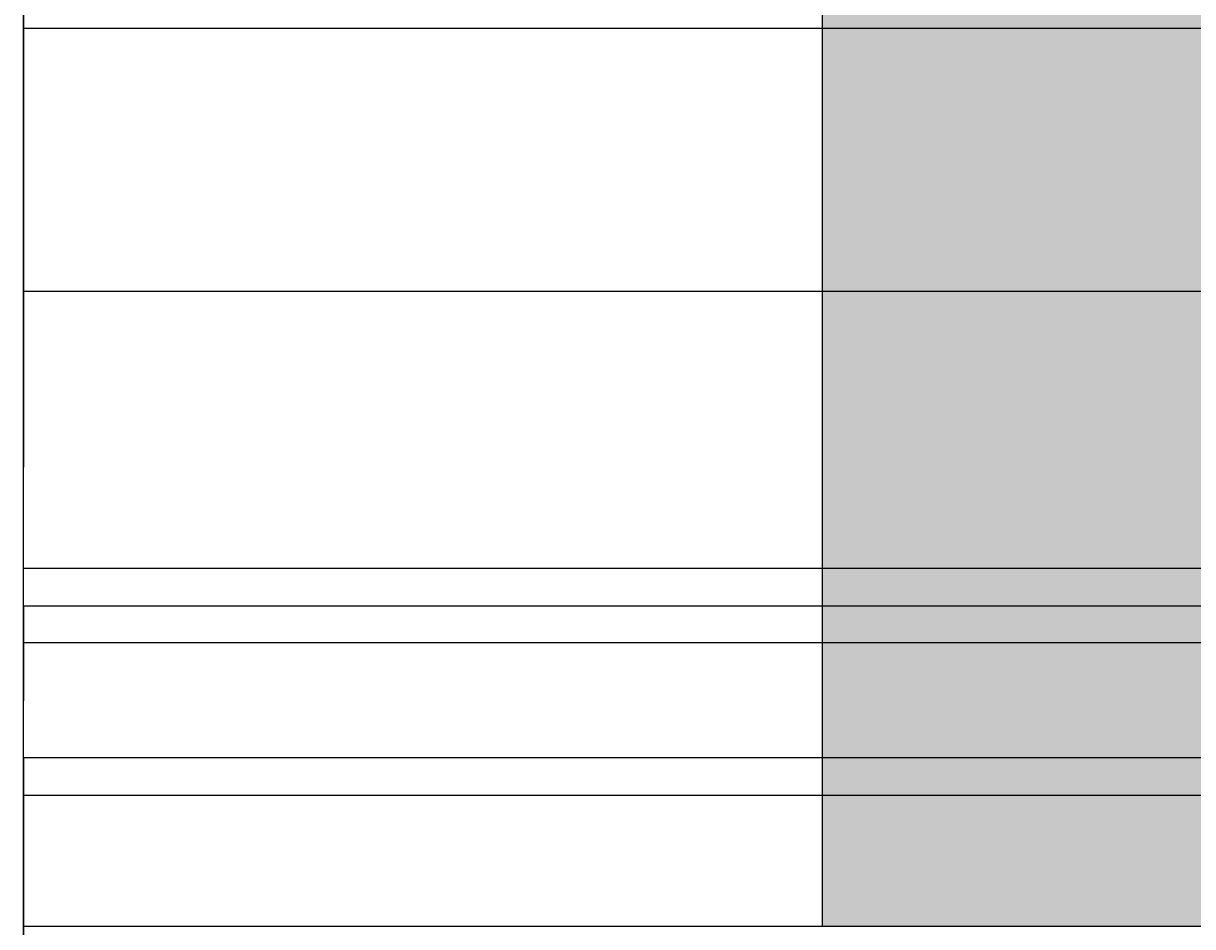
# Model space of a CAD drawing. Units: inches. Extents: x 35362 to 73946, y 43607 to 67532.
# Tile 3 of 134: x 35362 to 37937, y 46919 to 48909. Entities that reach past the tile are written whole.
import ezdxf

# ---------------------------------------------------------------- set-up
doc = ezdxf.new("R2010")
doc.units = ezdxf.units.IN
doc.header["$MEASUREMENT"] = 0
for name, color, linetype, lineweight in [('A-ANNO-DIMS', 2, 'Continuous', 18), ('E-SYMB', 1, 'Continuous', 25), ('E-SYMB-PATT', 1, 'Continuous', 13)]:
    doc.layers.add(name, color=color, linetype=linetype, lineweight=lineweight)
doc.styles.get("Standard").update_dxf_attribs({"font": 'arial.ttf'})
doc.dimstyles.get("Standard").update_dxf_attribs({"dimtxt": 0.18, "dimasz": 0.18, "dimexe": 0.18, "dimexo": 0.0625, "dimgap": 0.09, "dimtad": 0, "dimtih": 1, "dimtoh": 1, "dimdec": 4, "dimzin": 0, "dimdsep": 46, "dimtxsty": 'Standard', "dimcen": 0.09, "dimadec": 0, "dimazin": 0, "dimtfac": 1, "dimtdec": 4, "dimtofl": 0, "dimtmove": 0, "dimatfit": 3, "dimfxl": 1, "dimtolj": 1, "dimtzin": 0, "dimarcsym": 0})

# ---------------------------------------------------------------- blocks, each defined once
blk = doc.blocks.new('*D16')
at = {"layer": 'A-ANNO-DIMS', "color": 0, "lineweight": -2, "transparency": 16777216}
for p, q in [((37121.9, 49689.8), (35361.8, 49689.8)), ((35361.9, 49689.7), (35361.9, 48304.8)), ((35361.9, 46919.6), (35361.9, 48304.4)), ((37121.9, 46919.4), (35361.8, 46919.4))]:
    blk.add_line(p, q, dxfattribs=at)
at = {"layer": 'A-ANNO-DIMS', "color": 0, "transparency": 16777216}
for points in [[(35361.9, 49689.7), (35362, 49689.7), (35361.9, 49689.8)], [(35361.9, 46919.6), (35362, 46919.6), (35361.9, 46919.4)]]:
    blk.add_solid(points, dxfattribs=at)
at = {"layer": 'Defpoints', "color": 0, "transparency": 16777216}
for p in [(37121.9, 49689.8), (35361.9, 46919.4), (37121.9, 46919.4)]:
    blk.add_point(p, dxfattribs=at)
at = {"layer": 'A-ANNO-DIMS', "color": 0, "transparency": 16777216, "insert": (35361.9, 48304.6), "char_height": 0.18, "attachment_point": 5}
blk.add_mtext('\\A1;2770.5', dxfattribs=at)
blk = doc.blocks.new('*D43')
at = {"layer": 'A-ANNO-DIMS', "color": 0, "lineweight": -2, "transparency": 16777216}
for p, q in [((62004.7, 47625.2), (35361.8, 47625.2)), ((35361.9, 47625), (35361.9, 47416.9)), ((35361.9, 47208.4), (35361.9, 47416.5)), ((62004.7, 47208.2), (35361.8, 47208.2))]:
    blk.add_line(p, q, dxfattribs=at)
at = {"layer": 'A-ANNO-DIMS', "color": 0, "transparency": 16777216}
for points in [[(35361.9, 47625), (35362, 47625), (35361.9, 47625.2)], [(35361.9, 47208.4), (35362, 47208.4), (35361.9, 47208.2)]]:
    blk.add_solid(points, dxfattribs=at)
at = {"layer": 'Defpoints', "color": 0, "transparency": 16777216}
for p in [(62004.7, 47625.2), (35361.9, 47208.2), (62004.7, 47208.2)]:
    blk.add_point(p, dxfattribs=at)
at = {"layer": 'A-ANNO-DIMS', "color": 0, "transparency": 16777216, "insert": (35361.9, 47416.7), "char_height": 0.18, "attachment_point": 5}
blk.add_mtext('\\A1;416.9', dxfattribs=at)
blk = doc.blocks.new('*D67')
at = {"layer": 'A-ANNO-DIMS', "color": 0, "lineweight": -2, "transparency": 16777216}
for p, q in [((56873.5, 53351.5), (35361.8, 53351.5)), ((35361.9, 53351.3), (35361.9, 49400.9)), ((35361.9, 45450.1), (35361.9, 49400.5)), ((53793.6, 45449.9), (35361.8, 45449.9))]:
    blk.add_line(p, q, dxfattribs=at)
at = {"layer": 'A-ANNO-DIMS', "color": 0, "transparency": 16777216}
for points in [[(35361.9, 53351.3), (35362, 53351.3), (35361.9, 53351.5)], [(35361.9, 45450.1), (35362, 45450.1), (35361.9, 45449.9)]]:
    blk.add_solid(points, dxfattribs=at)
at = {"layer": 'Defpoints', "color": 0, "transparency": 16777216}
for p in [(35361.9, 53351.5), (56873.6, 53351.5), (53793.6, 45449.9)]:
    blk.add_point(p, dxfattribs=at)
at = {"layer": 'A-ANNO-DIMS', "color": 0, "transparency": 16777216, "insert": (35361.9, 49400.7), "char_height": 0.18, "attachment_point": 5}
blk.add_mtext('\\A1;7901.6', dxfattribs=at)
blk = doc.blocks.new('*D87')
at = {"layer": 'A-ANNO-DIMS', "color": 0, "lineweight": -2, "transparency": 16777216}
for p, q in [((52362.5, 48318.3), (35361.8, 48318.3)), ((35361.9, 48318.1), (35361.9, 47931.4)), ((35361.9, 47544.3), (35361.9, 47931)), ((52362.5, 47544.1), (35361.8, 47544.1))]:
    blk.add_line(p, q, dxfattribs=at)
at = {"layer": 'A-ANNO-DIMS', "color": 0, "transparency": 16777216}
for points in [[(35361.9, 48318.1), (35362, 48318.1), (35361.9, 48318.3)], [(35361.9, 47544.3), (35362, 47544.3), (35361.9, 47544.1)]]:
    blk.add_solid(points, dxfattribs=at)
at = {"layer": 'Defpoints', "color": 0, "transparency": 16777216}
for p in [(35361.9, 48318.3), (52362.6, 48318.3), (52362.6, 47544.1)]:
    blk.add_point(p, dxfattribs=at)
at = {"layer": 'A-ANNO-DIMS', "color": 0, "transparency": 16777216, "insert": (35361.9, 47931.2), "char_height": 0.18, "attachment_point": 5}
blk.add_mtext('\\A1;774.1', dxfattribs=at)
blk = doc.blocks.new('*D89')
at = {"layer": 'A-ANNO-DIMS', "color": 0, "lineweight": -2, "transparency": 16777216}
for p, q in [((53707.7, 48897.7), (35361.8, 48897.7)), ((35361.9, 48897.6), (35361.9, 48303.2)), ((35361.9, 47708.4), (35361.9, 48302.8)), ((53707.7, 47708.2), (35361.8, 47708.2))]:
    blk.add_line(p, q, dxfattribs=at)
at = {"layer": 'A-ANNO-DIMS', "color": 0, "transparency": 16777216}
for points in [[(35361.9, 48897.6), (35362, 48897.6), (35361.9, 48897.7)], [(35361.9, 47708.4), (35362, 47708.4), (35361.9, 47708.2)]]:
    blk.add_solid(points, dxfattribs=at)
at = {"layer": 'Defpoints', "color": 0, "transparency": 16777216}
for p in [(53707.8, 48897.7), (35361.9, 47708.2), (53707.8, 47708.2)]:
    blk.add_point(p, dxfattribs=at)
at = {"layer": 'A-ANNO-DIMS', "color": 0, "transparency": 16777216, "insert": (35361.9, 48303), "char_height": 0.18, "attachment_point": 5}
blk.add_mtext('\\A1;1189.5', dxfattribs=at)
blk = doc.blocks.new('*D90')
at = {"layer": 'A-ANNO-DIMS', "color": 0, "lineweight": -2, "transparency": 16777216}
for p, q in [((53707.7, 47291.3), (35361.8, 47291.3)), ((35361.9, 47291.1), (35361.9, 46710.3)), ((35361.9, 46129.1), (35361.9, 46709.9)), ((53793.6, 46128.9), (35361.8, 46128.9))]:
    blk.add_line(p, q, dxfattribs=at)
at = {"layer": 'A-ANNO-DIMS', "color": 0, "transparency": 16777216}
for points in [[(35361.9, 47291.1), (35362, 47291.1), (35361.9, 47291.3)], [(35361.9, 46129.1), (35362, 46129.1), (35361.9, 46128.9)]]:
    blk.add_solid(points, dxfattribs=at)
at = {"layer": 'Defpoints', "color": 0, "transparency": 16777216}
for p in [(53707.8, 47291.3), (35361.9, 46128.9), (53793.6, 46128.9)]:
    blk.add_point(p, dxfattribs=at)
at = {"layer": 'A-ANNO-DIMS', "color": 0, "transparency": 16777216, "insert": (35361.9, 46710.1), "char_height": 0.18, "attachment_point": 5}
blk.add_mtext('\\A1;1162.4', dxfattribs=at)

msp = doc.modelspace()

# ---------------------------------------------------------------- hatches: boundary and pattern name
at = {"layer": 'E-SYMB-PATT'}
h = msp.add_hatch(color=256, dxfattribs=at)
h.dxf.hatch_style = 1
h.paths.add_polyline_path([(39894.84, 49689.843), (37121.949, 49689.843), (37121.949, 46919.381), (39894.84, 46919.381)])

# ---------------------------------------------------------------- linework, layer by layer
at = {"layer": 'E-SYMB'}
msp.add_lwpolyline([(37121.949, 49689.843), (39894.84, 49689.843), (39894.84, 46919.381), (37121.949, 46919.381)], close=True, dxfattribs=at)

# ---------------------------------------------------------------- dimensions: what is measured, and where the dimension line sits
at = {"layer": 'A-ANNO-DIMS'}
for base, p1, p2, picture, middle in [((35361.949, 53351.529), (53793.638, 45449.894), (56873.602, 53351.529), '*D67', (35361.949, 49400.712)), ((35361.949, 46919.381), (37121.949, 49689.843), (37121.949, 46919.381), '*D16', (35361.949, 48304.612)), ((35361.949, 47708.216), (53707.781, 48897.738), (53707.781, 47708.216), '*D89', (35361.949, 48302.977)), ((35361.949, 48318.269), (52362.557, 47544.134), (52362.557, 48318.269), '*D87', (35361.949, 47931.201)), ((35361.949, 47208.25), (62004.728, 47625.181), (62004.728, 47208.25), '*D43', (35361.949, 47416.715)), ((35361.949, 46128.878), (53707.781, 47291.285), (53793.638, 46128.878), '*D90', (35361.949, 46710.081))]:
    dim = msp.add_linear_dim(base=base, p1=p1, p2=p2, angle=90, dimstyle='Standard', override={"dimdec": 1, "dimlfac": 1, "dimrnd": 0, "dimzin": 0, "dimdsep": 46, "dimlunit": 2}, dxfattribs=at)
    dim.commit()
    dim.dimension.update_dxf_attribs({"geometry": picture, "text_midpoint": middle})

doc.saveas('drawing.dxf')
